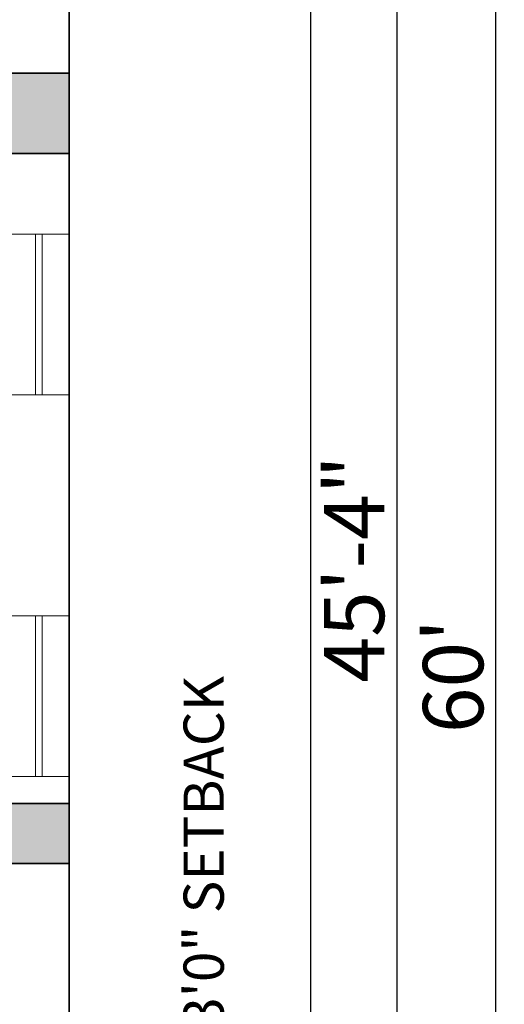
# Model space of a CAD drawing. Units: inches. Extents: x 3321 to 5237, y 11 to 1752.
# Tile 11 of 43: x 3793 to 3866, y 1298 to 1445. Entities that reach past the tile are written whole.
import ezdxf

# ---------------------------------------------------------------- set-up
doc = ezdxf.new("R2010")
doc.units = ezdxf.units.IN
for name, color, linetype, lineweight in [('A-ANNO-DIMS', 2, 'Continuous', 18), ('A-ANNO-TEXT', 7, 'Continuous', 18), ('A-COLS', 1, 'Continuous', 35), ('A-GLAZ', 5, 'Continuous', 18), ('A-WALL', 7, 'Continuous', 35), ('C-PROP', 7, 'Continuous', 30)]:
    doc.layers.add(name, color=color, linetype=linetype, lineweight=lineweight)
doc.styles.get("Standard").update_dxf_attribs({"font": 'arial.ttf'})
doc.dimstyles.new('ISO-25', dxfattribs={"dimtxt": 9, "dimasz": 2.5, "dimexe": 1.25, "dimexo": 0.625, "dimtad": 1, "dimdec": 1, "dimlunit": 3, "dimtxsty": 'Standard', "dimcen": 2.5, "dimclrd": 4, "dimclre": 4, "dimclrt": 256, "dimadec": 0, "dimazin": 0, "dimtfac": 1, "dimtdec": 1, "dimtmove": 0, "dimatfit": 3, "dimfxl": 1, "dimarcsym": 0})

# ---------------------------------------------------------------- blocks, each defined once
blk = doc.blocks.new('*D42')
at = {"layer": 'A-ANNO-DIMS', "color": 0, "lineweight": -2, "transparency": 16777216}
for p, q in [((3837.31, 1635.34), (3850.8, 1635.34)), ((3849.55, 1632.84), (3849.55, 1093.84)), ((3837.31, 1091.34), (3850.8, 1091.34))]:
    blk.add_line(p, q, dxfattribs=at)
at = {"layer": 'A-ANNO-DIMS', "color": 0, "transparency": 16777216}
for points in [[(3849.13, 1632.84), (3849.96, 1632.84), (3849.55, 1635.34)], [(3849.13, 1093.84), (3849.96, 1093.84), (3849.55, 1091.34)]]:
    blk.add_solid(points, dxfattribs=at)
at = {"layer": 'Defpoints', "color": 0, "transparency": 16777216}
for p in [(3836.69, 1635.34), (3836.69, 1091.34), (3849.55, 1091.34)]:
    blk.add_point(p, dxfattribs=at)
at = {"layer": 'A-ANNO-DIMS', "color": 0, "transparency": 16777216, "insert": (3844.35, 1363.34), "char_height": 9, "attachment_point": 5, "rotation": 90}
blk.add_mtext('45\'-4"', dxfattribs=at)
blk = doc.blocks.new('*D47')
at = {"layer": 'A-ANNO-DIMS', "color": 0, "lineweight": -2, "transparency": 16777216}
for p, q in [((3837.31, 1707.34), (3865.6, 1707.34)), ((3864.35, 989.84), (3864.35, 1704.84)), ((3837.31, 987.34), (3865.6, 987.34))]:
    blk.add_line(p, q, dxfattribs=at)
at = {"layer": 'A-ANNO-DIMS', "color": 0, "transparency": 16777216}
for points in [[(3863.93, 1704.84), (3864.76, 1704.84), (3864.35, 1707.34)], [(3863.93, 989.84), (3864.76, 989.84), (3864.35, 987.34)]]:
    blk.add_solid(points, dxfattribs=at)
at = {"layer": 'Defpoints', "color": 0, "transparency": 16777216}
for p in [(3836.69, 1707.34), (3864.35, 1707.34), (3836.69, 987.34)]:
    blk.add_point(p, dxfattribs=at)
at = {"layer": 'A-ANNO-DIMS', "color": 0, "transparency": 16777216, "insert": (3859.13, 1347.34), "char_height": 9, "attachment_point": 5, "rotation": 90}
blk.add_mtext("60'", dxfattribs=at)
blk = doc.blocks.new('COL-9X12-FURN-PLAN')
h = blk.add_hatch(color=256)
h.dxf.hatch_style = 1
h.paths.add_polyline_path([(0, 12), (0, 0), (9, 0), (9, 12)])
blk.add_lwpolyline([(0, 0), (9, 0), (9, 12), (0, 12)], close=True)
blk = doc.blocks.new('COL-9X9-FURN-PLAN')
h = blk.add_hatch(color=256)
h.dxf.hatch_style = 1
h.paths.add_polyline_path([(9, 9), (0, 9), (0, 0), (9, 0)])
blk.add_lwpolyline([(0, 0), (9, 0), (9, 9), (0, 9)], close=True)
blk = doc.blocks.new('WIN-24IN-9IN-WALL')
for p, q in [((9, 24), (0, 24)), ((4, 24), (4, 0)), ((5, 24), (5, 0)), ((9, 0), (0, 0))]:
    blk.add_line(p, q)
blk = doc.blocks.new('PROPERTY-40X60FT')
blk.add_line((480, 720), (480, 0))

msp = doc.modelspace()

# ---------------------------------------------------------------- linework, layer by layer
at = {"layer": 'A-WALL'}
msp.add_line((3800.69, 1635.34), (3800.69, 1091.34), dxfattribs=at)

# ---------------------------------------------------------------- block references
at = {"layer": 'A-COLS'}
for name, p in [('COL-9X12-FURN-PLAN', (3791.69, 1425.34)), ('COL-9X9-FURN-PLAN', (3791.69, 1319.34))]:
    msp.add_blockref(name, p, dxfattribs=at)
at = {"layer": 'A-GLAZ'}
for p in [(3791.69, 1389.34), (3791.69, 1332.34)]:
    msp.add_blockref('WIN-24IN-9IN-WALL', p, dxfattribs=at)
at = {"layer": 'C-PROP'}
msp.add_blockref('PROPERTY-40X60FT', (3356.69, 987.34), dxfattribs=at)

# ---------------------------------------------------------------- texts
at = {"layer": 'A-ANNO-TEXT', "insert": (3817.76, 1294.84), "char_height": 6, "attachment_point": 1, "rotation": 90}
msp.add_mtext_dynamic_manual_height_columns('3\'0" SETBACK', width=97.3114, gutter_width=25, heights=[0], dxfattribs=at)

# ---------------------------------------------------------------- dimensions: what is measured, and where the dimension line sits
at = {"layer": 'A-ANNO-DIMS'}
for base, p1, p2, angle, override, picture, middle in [((3864.35, 1707.34), (3836.69, 987.34), (3836.69, 1707.34), 270, {"dimclrd": 0, "dimclre": 0, "dimclrt": 0}, '*D47', (3859.13, 1347.34)), ((3849.55, 1091.34), (3836.69, 1635.34), (3836.69, 1091.34), 90, {"dimclrd": 0, "dimclre": 0, "dimclrt": 0, "dimtmove": 1}, '*D42', (3844.35, 1363.34))]:
    dim = msp.add_linear_dim(base=base, p1=p1, p2=p2, angle=angle, dimstyle='ISO-25', override=override, dxfattribs=at)
    dim.commit()
    dim.dimension.update_dxf_attribs({"geometry": picture, "text_midpoint": middle})

doc.saveas('drawing.dxf')
